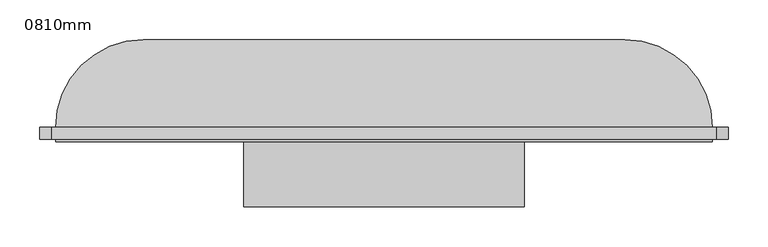
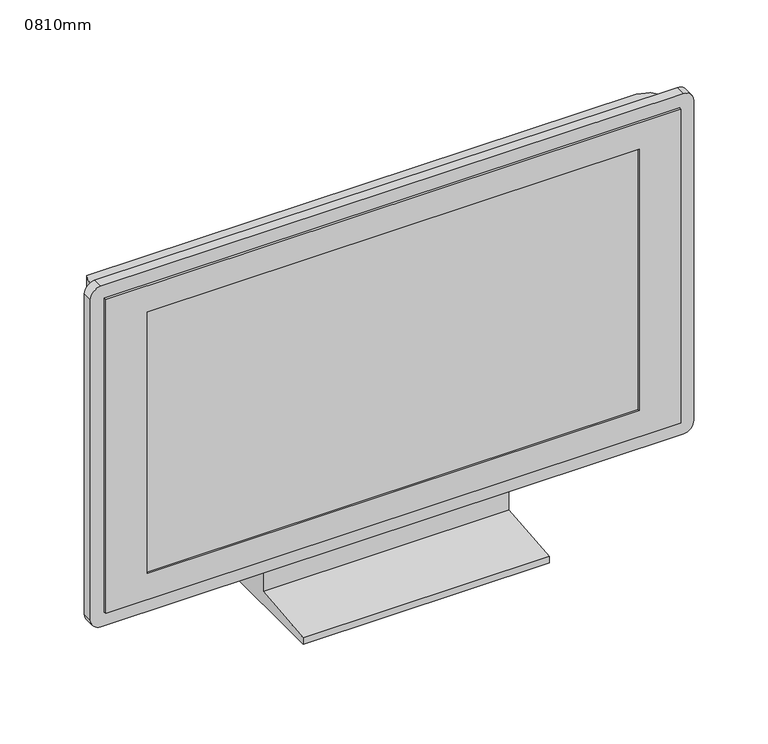
"""IFC4 building model written with IfcOpenShell, lengths in millimetres: furniture geometry, 0810mm."""

from ifc_helpers import new_model, si_unit, point, frame, frame_2d, origin, place, context, project, spatial, polyline, circle_curve, ellipse_curve, trimmed, segment, composite_curve, outline, extrude, faceted_brep, source, transform, mapped, element, save
from ifc_brep_helpers import plane_surface, cylinder_surface, advanced_brep


def furniture_0810mm_51289c3c(model_context):
    return source(origin(), model_context, "Body", "SolidModel", [
        advanced_brep(
        [(-416.9248214, -51.4613764, 80.0), (409.0357931, -51.4613764, 80.0), (409.0357931, -51.4613764, 557.1392838), (-416.9248214, -51.4613764, 557.1392838), (299.0357931, 58.5386236, 80.0), (-306.9248214, 58.5386236, 80.0), (-306.9248214, 58.5386236, 447.1392838), (299.0357931, 58.5386236, 447.1392838)],
        [
            (0, 1),
            (1, 2),
            (2, 3),
            (3, 0),
            (4, 5),
            (5, 6),
            (6, 7),
            (7, 4),
            (0, 5, circle_curve(frame((-306.9248214, -51.4613764, 80.0), z_axis=(0.0, 0.0, -1.0), x_axis=(-1.0, 0.0, 0.0)), 110.0)),
            (4, 1, circle_curve(frame((299.0357931, -51.4613764, 80.0), z_axis=(0.0, 0.0, -1.0), x_axis=(1.0, 0.0, 0.0)), 110.0)),
            (7, 2, ellipse_curve(frame((299.0357931, -51.4613764, 447.1392838), z_axis=(0.7071067811865475, 0.0, -0.7071067811865475), x_axis=(0.7071067811865474, 0.0, 0.7071067811865476)), 155.5634919, 110.0)),
            (6, 3, ellipse_curve(frame((-306.9248214, -51.4613764, 447.1392838), z_axis=(0.7071067811865475, 0.0, 0.7071067811865475), x_axis=(-0.7071067811865476, 0.0, 0.7071067811865474)), 155.5634919, 110.0)),
        ],
        [
            plane_surface(frame((-416.9248214, -51.4613764, 557.1392838), z_axis=(0.0, -1.0, 0.0), x_axis=(-1.0, 0.0, 0.0))),
            plane_surface(frame((-416.9248214, 58.5386236, 557.1392838), z_axis=(0.0, 1.0, 0.0), x_axis=(1.0, 0.0, 0.0))),
            plane_surface(frame((-416.9248214, -51.4613764, 80.0), z_axis=(0.0, 0.0, -1.0), x_axis=(0.0, 1.0, 0.0))),
            cylinder_surface(frame((299.0357931, -51.4613764, 80.0), z_axis=(0.0, 0.0, 1.0), x_axis=(1.0, 0.0, 0.0)), 110.0),
            cylinder_surface(frame((409.0357931, -51.4613764, 447.1392838), z_axis=(-1.0, 0.0, 0.0), x_axis=(0.0, 0.0, 1.0)), 110.0),
            cylinder_surface(frame((-306.9248214, -51.4613764, 557.1392838), z_axis=(0.0, 0.0, -1.0), x_axis=(-1.0, 0.0, 0.0)), 110.0),
        ],
        [
            (0, [[1, 2, 3, 4]]),
            (1, [[5, 6, 7, 8]]),
            (2, [[-1, 9, -5, 10]]),
            (3, [[11, -2, -10, -8]]),
            (4, [[-11, -7, 12, -3]]),
            (5, [[-12, -6, -9, -4]]),
        ],
    ),
        extrude(outline(composite_curve([segment(polyline([(577.1392838, 414.0357931), (577.1392838, -421.9248214)]), True, "CONTINUOUS"), segment(trimmed(circle_curve(frame_2d((562.1392838, -421.9248214)), 15.0), [point((577.1392838, -421.9248214))], [point((562.1392838, -436.9248214))], False, "CARTESIAN"), True, "CONTINUOUS"), segment(polyline([(562.1392838, -436.9248214), (75.0, -436.9248214)]), True, "CONTINUOUS"), segment(trimmed(circle_curve(frame_2d((75.0, -421.9248214)), 15.0), [point((75.0, -436.9248214))], [point((60.0, -421.9248214))], False, "CARTESIAN"), True, "CONTINUOUS"), segment(polyline([(60.0, -421.9248214), (60.0, 414.0357931)]), True, "CONTINUOUS"), segment(trimmed(circle_curve(frame_2d((75.0, 414.0357931)), 15.0), [point((60.0, 414.0357931))], [point((75.0, 429.0357931))], False, "CARTESIAN"), True, "CONTINUOUS"), segment(polyline([(75.0, 429.0357931), (562.1392838, 429.0357931)]), True, "CONTINUOUS"), segment(trimmed(circle_curve(frame_2d((562.1392838, 414.0357931)), 15.0), [point((562.1392838, 429.0357931))], [point((577.1392838, 414.0357931))], False, "CARTESIAN"), True, "CONTINUOUS")], self_intersect=False), holes=[polyline([(557.1392838, 409.0357931), (80.0, 409.0357931), (80.0, -416.9248214), (557.1392838, -416.9248214), (557.1392838, 409.0357931)])]), frame((0.0, -66.4613764, 0.0), z_axis=(0.0, 1.0, 0.0), x_axis=(0.0, 0.0, 1.0)), (0.0, 0.0, 1.0), 15.0),
        faceted_brep([(409.0357931, -69.4613764, 557.1392838), (-416.9248214, -69.4613764, 557.1392838), (-416.9248214, -69.4613764, 80.0), (409.0357931, -69.4613764, 80.0), (-356.9248214, -69.4613764, 517.1392838), (349.0357931, -69.4613764, 517.1392838), (349.0357931, -69.4613764, 120.0), (-356.9248214, -69.4613764, 120.0), (409.0357931, -51.4613764, 557.1392838), (409.0357931, -51.4613764, 80.0), (-416.9248214, -51.4613764, 80.0), (-416.9248214, -51.4613764, 557.1392838), (-356.9248214, -66.4613764, 517.1392838), (-356.9248214, -66.4613764, 120.0), (349.0357931, -66.4613764, 120.0), (349.0357931, -66.4613764, 517.1392838)], [[[0, 1, 2, 3], [4, 5, 6, 7]], [[8, 9, 10, 11]], [[1, 0, 8, 11]], [[2, 1, 11, 10]], [[3, 2, 10, 9]], [[0, 3, 9, 8]], [[12, 13, 14, 15]], [[12, 15, 5, 4]], [[15, 14, 6, 5]], [[14, 13, 7, 6]], [[13, 12, 4, 7]]]),
        extrude(outline(polyline([(-51.4613764, 80.0), (-1.4613764, 80.0), (48.5386236, 0.0), (-151.4613764, 0.0), (-151.4613764, 10.0), (-51.4613764, 20.0), (-51.4613764, 80.0)])), frame((-180.4346678, 0.0, 0.0), z_axis=(1.0, 0.0, 0.0), x_axis=(0.0, 1.0, 0.0)), (0.0, 0.0, 1.0), 352.9803073),
    ])


if __name__ == "__main__":
    model = new_model("IFC4")
    model_context = context("Model", 3, world=origin())
    ifc_project = project(units=[si_unit("LENGTHUNIT", "METRE", prefix="MILLI")], contexts=[model_context])
    site = spatial("IfcSite", under=ifc_project)
    building = spatial("IfcBuilding", under=site)
    placement = place(None, origin())
    furniture_0810mm_shape = furniture_0810mm_51289c3c(model_context)
    element("IfcFurniture", 1, ObjectType="0810mm", at=placement, inside=building, context=model_context, shape_type="MappedRepresentation", body=[
        mapped(furniture_0810mm_shape, transform((0.0, 0.0, 0.0), x_axis=(1.0, 0.0, 0.0), y_axis=(0.0, 1.0, 0.0), z_axis=(0.0, 0.0, 1.0))),
    ])
    save(model, "model.ifc")

# Revit data of these elements
# Type "0810mm"
#   SinAng = 0.001609 ft
#   L = 2.316144 ft
#   H = 1.30295 ft
#   Thickness = 0.360892 ft
#   Diagonal = 2.65748 ft
#   CosAng = 0.002859 ft
#   Stand [instance default] = yes
#   Default Elevation = 0
# Element 1 (IfcFurniture, "0810mm")
#   Materials on its faces: "TV - Black", "TV - Glass", "TV - Screen"
# Materials
#   "TV - Black": colour RGB 49 49 49, transparency 0
#   "TV - Glass": colour RGB 157 157 157, transparency 0.9
#   "TV - Screen": colour RGB 0 0 0, transparency 0
